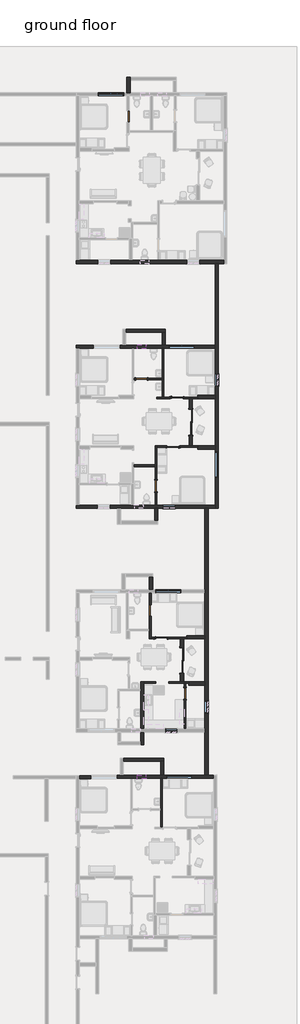
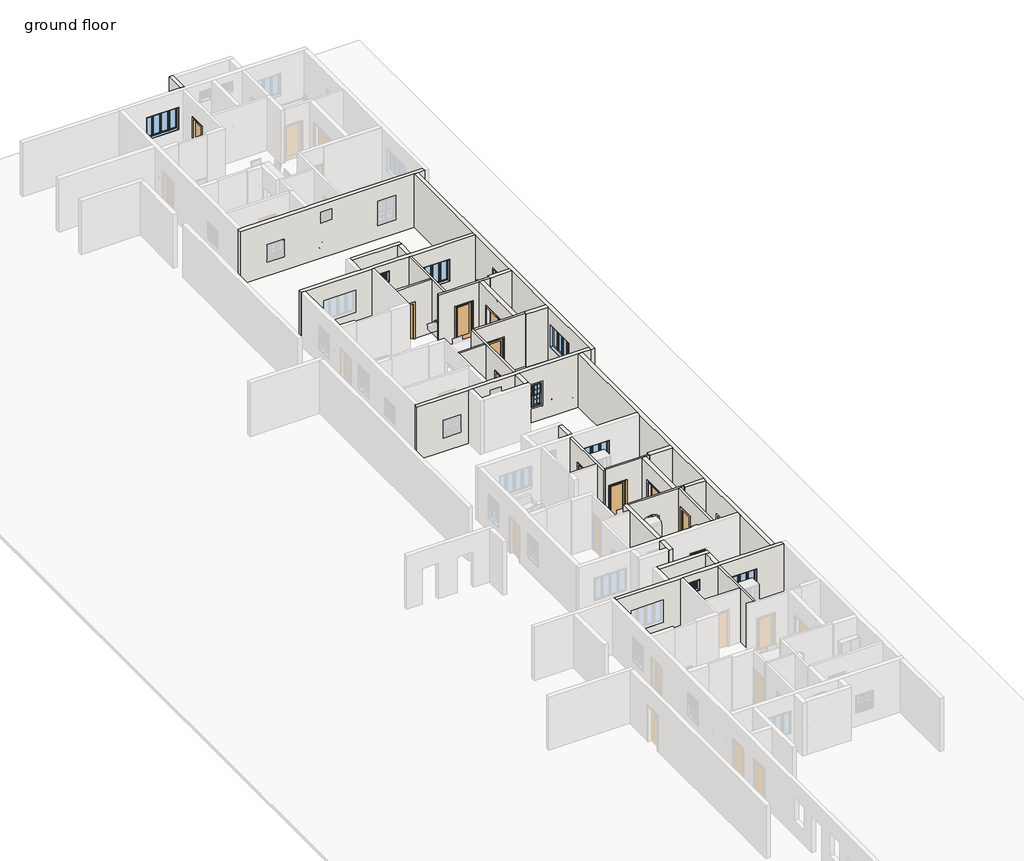
# One storey, part 9 of 16: 32 walls, 11 windows, 10 doors.
"""IFC4 building model written with IfcOpenShell, lengths in millimetres."""

from ifc_helpers import new_model, si_unit, point, frame, origin, place, context, project, spatial, polyline, ellipse_curve, trimmed, outline, extrude, faceted_brep, transform, mapped, element, save
from ifc_brep_helpers import plane_surface, extruded_surface, advanced_brep
from components import door_d4d75d1e, door_3c6ab76a, door_377e7377, door_38851409, door_d141acb4, window_ced37e8f, window_5487fb6d, window_f2d8fef0, window_45970670

model = new_model("IFC4")

# Units and contexts
model_context = context("Model", 3, world=origin())
ifc_project = project(units=[si_unit("LENGTHUNIT", "METRE", prefix="MILLI")], contexts=[model_context])

# Site, building, storey
site = spatial("IfcSite", under=ifc_project)
building = spatial("IfcBuilding", under=site)
storey = spatial("IfcBuildingStorey", under=building, Name="ground floor", Elevation=609.6)

# Doors
placement = place(None, origin())
door_shape = door_d4d75d1e(model_context)
element("IfcDoor", 1, ObjectType="Door-Double-Sliding : 72\" x 84\"", at=placement, inside=storey, context=model_context, shape_type="MappedRepresentation", body=[
    mapped(door_shape, transform((67382.9312819, 27142.5650652, 609.6), x_axis=(0.0, -1.0, 0.0), y_axis=(1.0, 0.0, 0.0), z_axis=(0.0, 0.0, 1.0))),
])
element("IfcDoor", 2, ObjectType="Door-Double-Sliding : 72\" x 84\"", at=placement, inside=storey, context=model_context, shape_type="MappedRepresentation", body=[
    mapped(door_shape, transform((66760.6312819, 10200.7650652, 609.6), x_axis=(0.0, -1.0, 0.0), y_axis=(1.0, 0.0, 0.0), z_axis=(0.0, 0.0, 1.0))),
])
door_2_shape = door_3c6ab76a(model_context)
element("IfcDoor", 3, ObjectType="Door-Interior-Single-1_Panel-Wood : 36\" x 84\"", at=placement, inside=storey, context=model_context, shape_type="MappedRepresentation", body=[
    mapped(door_2_shape, transform((66522.5062819, 28879.2900652, 609.6), x_axis=(1.0, 0.0, 0.0), y_axis=(0.0, 1.0, 0.0), z_axis=(0.0, 0.0, 1.0))),
])
element("IfcDoor", 4, ObjectType="Door-Interior-Single-1_Panel-Wood : 36\" x 84\"", at=placement, inside=storey, context=model_context, shape_type="MappedRepresentation", body=[
    mapped(door_2_shape, transform((66281.2062819, 25405.8400652, 609.6), x_axis=(-1.0, 0.0, 0.0), y_axis=(0.0, -1.0, 0.0), z_axis=(0.0, 0.0, 1.0))),
])
element("IfcDoor", 5, ObjectType="Door-Interior-Single-1_Panel-Wood : 36\" x 84\"", at=placement, inside=storey, context=model_context, shape_type="MappedRepresentation", body=[
    mapped(door_2_shape, transform((65395.3812819, 11785.0900652, 609.6), x_axis=(1.0, 0.0, 0.0), y_axis=(0.0, 1.0, 0.0), z_axis=(0.0, 0.0, 1.0))),
])
door_3_shape = door_377e7377(model_context)
element("IfcDoor", 6, ObjectType="Single-Flush : 32\" x 84\"", at=placement, inside=storey, context=model_context, shape_type="MappedRepresentation", body=[
    mapped(door_3_shape, transform((63051.0711425, 48883.2273256, 609.6), x_axis=(0.0, -1.0, 0.0), y_axis=(1.0, 0.0, 0.0), z_axis=(0.0, 0.0, 1.0))),
])
door_4_shape = door_38851409(model_context)
element("IfcDoor", 7, ObjectType="Single-Flush : 32\" x 84\"", at=placement, inside=storey, context=model_context, shape_type="MappedRepresentation", body=[
    mapped(door_4_shape, transform((67097.1812819, 7857.6150652, 609.6), x_axis=(0.0, 1.0, 0.0), y_axis=(-1.0, 0.0, 0.0), z_axis=(0.0, 0.0, 1.0))),
])
element("IfcDoor", 8, ObjectType="Single-Flush : 32\" x 84\"", at=placement, inside=storey, context=model_context, shape_type="MappedRepresentation", body=[
    mapped(door_4_shape, transform((64633.3812819, 13734.5400652, 609.6), x_axis=(0.0, -1.0, 0.0), y_axis=(1.0, 0.0, 0.0), z_axis=(0.0, 0.0, 1.0))),
])
door_5_shape = door_d141acb4(model_context)
element("IfcDoor", 9, ObjectType="Single-Flush : 32\" x 84\"", at=placement, inside=storey, context=model_context, shape_type="MappedRepresentation", body=[
    mapped(door_5_shape, transform((64023.7812819, 30209.6150652, 609.6), x_axis=(1.0, 0.0, 0.0), y_axis=(0.0, 1.0, 0.0), z_axis=(0.0, 0.0, 1.0))),
])
element("IfcDoor", 10, ObjectType="Single-Flush : 32\" x 84\"", at=placement, inside=storey, context=model_context, shape_type="MappedRepresentation", body=[
    mapped(door_5_shape, transform((65052.4812819, 22592.7900652, 609.6), x_axis=(0.0, 1.0, 0.0), y_axis=(-1.0, 0.0, 0.0), z_axis=(0.0, 0.0, 1.0))),
])

# Walls
element("IfcWall", 11, ObjectType="Generic - 4.5\"", at=placement, inside=storey, context=model_context, shape_type="SweptSolid", body=[
    extrude(outline(polyline([(64995.3312819, 23992.9650652), (63471.3312819, 23992.9650652), (63471.3312819, 24107.2650652), (64995.3312819, 24107.2650652), (64995.3312819, 23992.9650652)])), frame((0.0, 0.0, 609.6), z_axis=(0.0, 0.0, 1.0), x_axis=(1.0, 0.0, 0.0)), (0.0, 0.0, 1.0), 3200.4),
])
element("IfcWall", 12, ObjectType="Generic - 4.5\"", at=placement, inside=storey, context=model_context, shape_type="Brep", body=[
    faceted_brep([(64995.3312819, 25466.1650652, 609.6), (64995.3312819, 24107.2650652, 609.6), (64995.3312819, 23992.9650652, 609.6), (64995.3312819, 22999.1900652, 609.6), (64995.3312819, 22999.1900652, 2743.2), (64995.3312819, 22186.3900652, 2743.2), (64995.3312819, 22186.3900652, 609.6), (64995.3312819, 21249.7650652, 609.6), (64995.3312819, 21249.7650652, 3810.0), (64995.3312819, 23992.9650652, 3810.0), (64995.3312819, 24107.2650652, 3810.0), (64995.3312819, 25466.1650652, 3810.0), (65109.6312819, 22999.1900652, 2743.2), (65109.6312819, 22999.1900652, 609.6), (65109.6312819, 25351.8650652, 609.6), (65109.6312819, 25466.1650652, 609.6), (65109.6312819, 25466.1650652, 3810.0), (65109.6312819, 25351.8650652, 3810.0), (65109.6312819, 21249.7650652, 3810.0), (65109.6312819, 21249.7650652, 609.6), (65109.6312819, 22186.3900652, 609.6), (65109.6312819, 22186.3900652, 2743.2)], [[[0, 1, 2, 3, 4, 5, 6, 7, 8, 9, 10, 11]], [[12, 13, 14, 15, 16, 17, 18, 19, 20, 21]], [[20, 19, 7, 6]], [[15, 14, 13, 3, 2, 1, 0]], [[11, 10, 9, 8, 18, 17, 16]], [[8, 7, 19, 18]], [[0, 11, 16, 15]], [[4, 3, 13, 12]], [[5, 4, 12, 21]], [[6, 5, 21, 20]]]),
])
element("IfcWall", 13, ObjectType="Generic - 4.5\"", at=placement, inside=storey, context=model_context, shape_type="Brep", body=[
    faceted_brep([(68017.0909667, 25351.8650652, 609.6), (68017.0909667, 25351.8650652, 3810.0), (65109.6312819, 25351.8650652, 3810.0), (65109.6312819, 25351.8650652, 609.6), (65798.6062819, 25351.8650652, 609.6), (65798.6062819, 25351.8650652, 2768.6), (66763.8062819, 25351.8650652, 2768.6), (66763.8062819, 25351.8650652, 609.6), (68017.0909667, 25466.1650652, 3810.0), (68017.0909667, 25466.1650652, 609.6), (67624.2312819, 25466.1650652, 609.6), (67395.6312819, 25466.1650652, 609.6), (66763.8062819, 25466.1650652, 609.6), (66763.8062819, 25466.1650652, 2768.6), (65798.6062819, 25466.1650652, 2768.6), (65798.6062819, 25466.1650652, 609.6), (65109.6312819, 25466.1650652, 609.6), (65109.6312819, 25466.1650652, 3810.0), (67395.6312819, 25466.1650652, 3810.0), (67624.2312819, 25466.1650652, 3810.0)], [[[0, 1, 2, 3, 4, 5, 6, 7]], [[8, 9, 10, 11, 12, 13, 14, 15, 16, 17, 18, 19]], [[3, 16, 15, 4]], [[9, 0, 7, 12, 11, 10]], [[1, 0, 9, 8]], [[2, 1, 8, 19, 18, 17]], [[3, 2, 17, 16]], [[14, 5, 4, 15]], [[5, 14, 13, 6]], [[6, 13, 12, 7]]]),
])
element("IfcWall", 14, ObjectType="Generic - 4.5\"", at=placement, inside=storey, context=model_context, shape_type="SweptSolid", body=[
    extrude(outline(polyline([(2743.2, 64430.1812819), (609.6, 64430.1812819), (609.6, 65477.9312819), (3810.0, 65477.9312819), (3810.0, 63471.3312819), (609.6, 63471.3312819), (609.6, 63617.3812819), (2743.2, 63617.3812819), (2743.2, 64430.1812819)])), frame((0.0, 30152.4650652, 0.0), z_axis=(0.0, 1.0, 0.0), x_axis=(0.0, 0.0, 1.0)), (0.0, 0.0, 1.0), 114.3),
])
element("IfcWall", 15, ObjectType="Generic - 4.5\"", at=placement, inside=storey, context=model_context, shape_type="Brep", body=[
    faceted_brep([(65477.9312819, 32400.3650652, 609.6), (65477.9312819, 30266.7650652, 609.6), (65477.9312819, 30152.4650652, 609.6), (65477.9312819, 28933.2650652, 609.6), (65477.9312819, 28933.2650652, 3810.0), (65477.9312819, 30152.4650652, 3810.0), (65477.9312819, 30266.7650652, 3810.0), (65477.9312819, 32400.3650652, 3810.0), (65592.2312819, 32400.3650652, 609.6), (65592.2312819, 32400.3650652, 3810.0), (65592.2312819, 28933.2650652, 3810.0), (65592.2312819, 28933.2650652, 609.6)], [[[0, 1, 2, 3, 4, 5, 6, 7]], [[8, 9, 10, 11]], [[3, 2, 1, 0, 8, 11]], [[7, 6, 5, 4, 10, 9]], [[0, 7, 9, 8]], [[4, 3, 11, 10]]]),
])
element("IfcWall", 16, ObjectType="Generic - 4.5\"", at=placement, inside=storey, context=model_context, shape_type="Brep", body=[
    faceted_brep([(68017.0909667, 28818.9650652, 609.6), (68017.0909667, 28818.9650652, 3810.0), (67624.2312819, 28818.9650652, 3810.0), (67395.6312819, 28818.9650652, 3810.0), (65109.6312819, 28818.9650652, 3810.0), (65109.6312819, 28818.9650652, 609.6), (66039.9062819, 28818.9650652, 609.6), (66039.9062819, 28818.9650652, 2768.6), (67005.1062819, 28818.9650652, 2768.6), (67005.1062819, 28818.9650652, 609.6), (67395.6312819, 28818.9650652, 609.6), (67624.2312819, 28818.9650652, 609.6), (68017.0909667, 28933.2650652, 3810.0), (68017.0909667, 28933.2650652, 609.6), (67005.1062819, 28933.2650652, 609.6), (67005.1062819, 28933.2650652, 2768.6), (66039.9062819, 28933.2650652, 2768.6), (66039.9062819, 28933.2650652, 609.6), (65592.2312819, 28933.2650652, 609.6), (65477.9312819, 28933.2650652, 609.6), (65109.6312819, 28933.2650652, 609.6), (65109.6312819, 28933.2650652, 3810.0), (65477.9312819, 28933.2650652, 3810.0), (65592.2312819, 28933.2650652, 3810.0)], [[[0, 1, 2, 3, 4, 5, 6, 7, 8, 9, 10, 11]], [[12, 13, 14, 15, 16, 17, 18, 19, 20, 21, 22, 23]], [[5, 20, 19, 18, 17, 6]], [[13, 0, 11, 10, 9, 14]], [[1, 0, 13, 12]], [[4, 3, 2, 1, 12, 23, 22, 21]], [[5, 4, 21, 20]], [[8, 15, 14, 9]], [[15, 8, 7, 16]], [[16, 7, 6, 17]]]),
])
element("IfcWall", 17, ObjectType="Generic - 4.5\"", at=placement, inside=storey, context=model_context, shape_type="Brep", body=[
    faceted_brep([(64576.2312819, 13328.1400652, 2743.2), (64576.2312819, 13328.1400652, 609.6), (64576.2312819, 12410.5650652, 609.6), (64576.2312819, 12296.2650652, 609.6), (64576.2312819, 11724.7650652, 609.6), (64576.2312819, 11724.7650652, 3810.0), (64576.2312819, 12296.2650652, 3810.0), (64576.2312819, 12410.5650652, 3810.0), (64576.2312819, 15001.3650652, 3810.0), (64576.2312819, 15001.3650652, 609.6), (64576.2312819, 14140.9400652, 609.6), (64576.2312819, 14140.9400652, 2743.2), (64690.5312819, 11724.7650652, 609.6), (64690.5312819, 11839.0650652, 609.6), (64690.5312819, 13328.1400652, 609.6), (64690.5312819, 13328.1400652, 2743.2), (64690.5312819, 14140.9400652, 2743.2), (64690.5312819, 14140.9400652, 609.6), (64690.5312819, 15001.3650652, 609.6), (64690.5312819, 15001.3650652, 3810.0), (64690.5312819, 11839.0650652, 3810.0), (64690.5312819, 11724.7650652, 3810.0)], [[[0, 1, 2, 3, 4, 5, 6, 7, 8, 9, 10, 11]], [[12, 13, 14, 15, 16, 17, 18, 19, 20, 21]], [[10, 9, 18, 17]], [[4, 3, 2, 1, 14, 13, 12]], [[8, 7, 6, 5, 21, 20, 19]], [[9, 8, 19, 18]], [[5, 4, 12, 21]], [[15, 14, 1, 0]], [[16, 15, 0, 11]], [[17, 16, 11, 10]]]),
])
element("IfcWall", 18, ObjectType="Generic - 4.5\"", at=placement, inside=storey, context=model_context, shape_type="Brep", body=[
    faceted_brep([(67216.0628293, 11724.7650652, 609.6), (67216.0628293, 11724.7650652, 3810.0), (67001.9312819, 11724.7650652, 3810.0), (66773.3312819, 11724.7650652, 3810.0), (64690.5312819, 11724.7650652, 3810.0), (64690.5312819, 11724.7650652, 609.6), (64912.7812819, 11724.7650652, 609.6), (64912.7812819, 11724.7650652, 2768.6), (65877.9812819, 11724.7650652, 2768.6), (65877.9812819, 11724.7650652, 609.6), (66773.3312819, 11724.7650652, 609.6), (67001.9312819, 11724.7650652, 609.6), (67216.0628293, 11839.0650652, 3810.0), (67216.0628293, 11839.0650652, 609.6), (65877.9812819, 11839.0650652, 609.6), (65877.9812819, 11839.0650652, 2768.6), (64912.7812819, 11839.0650652, 2768.6), (64912.7812819, 11839.0650652, 609.6), (64690.5312819, 11839.0650652, 609.6), (64690.5312819, 11839.0650652, 3810.0)], [[[0, 1, 2, 3, 4, 5, 6, 7, 8, 9, 10, 11]], [[12, 13, 14, 15, 16, 17, 18, 19]], [[5, 18, 17, 6]], [[13, 0, 11, 10, 9, 14]], [[1, 0, 13, 12]], [[4, 3, 2, 1, 12, 19]], [[5, 4, 19, 18]], [[8, 15, 14, 9]], [[15, 8, 7, 16]], [[16, 7, 6, 17]]]),
])
element("IfcWall", 19, ObjectType="Generic - 4.5\"", at=placement, inside=storey, context=model_context, shape_type="AdvancedBrep", body=[
    advanced_brep(
    [(65020.7312819, 8676.7650652, 2540.0), (65020.7312819, 8676.7650652, 609.6), (64182.5312819, 8676.7650652, 609.6), (64182.5312819, 8676.7650652, 3810.0), (66773.3312819, 8676.7650652, 3810.0), (67001.9312819, 8676.7650652, 3810.0), (67357.5312819, 8676.7650652, 3810.0), (67357.5312819, 8676.7650652, 609.6), (67001.9312819, 8676.7650652, 609.6), (66773.3312819, 8676.7650652, 609.6), (65935.1312819, 8676.7650652, 609.6), (65935.1312819, 8676.7650652, 2540.0), (64182.5312819, 8562.4650652, 609.6), (65020.7312819, 8562.4650652, 609.6), (65020.7312819, 8562.4650652, 2540.0), (65935.1312819, 8562.4650652, 2540.0), (65935.1312819, 8562.4650652, 609.6), (67040.0312819, 8562.4650652, 609.6), (67154.3312819, 8562.4650652, 609.6), (67357.5312819, 8562.4650652, 609.6), (67357.5312819, 8562.4650652, 3810.0), (67154.3312819, 8562.4650652, 3810.0), (67040.0312819, 8562.4650652, 3810.0), (64182.5312819, 8562.4650652, 3810.0)],
    [
        (0, 1),
        (1, 2),
        (2, 3),
        (3, 4),
        (4, 5),
        (5, 6),
        (6, 7),
        (7, 8),
        (8, 9),
        (9, 10),
        (10, 11),
        (11, 0, ellipse_curve(frame((65477.9312819, 8676.7650652, 2540.0), z_axis=(0.0, -1.0, 0.0), x_axis=(-1.0, 0.0, 0.0)), 457.2, 203.2)),
        (12, 13),
        (13, 14),
        (14, 15, ellipse_curve(frame((65477.9312819, 8562.4650652, 2540.0), z_axis=(0.0, 1.0, 0.0), x_axis=(-1.0, 0.0, 0.0)), 457.2, 203.2)),
        (15, 16),
        (16, 17),
        (17, 18),
        (18, 19),
        (19, 20),
        (20, 21),
        (21, 22),
        (22, 23),
        (23, 12),
        (1, 13),
        (12, 2),
        (7, 19),
        (16, 10),
        (3, 23),
        (20, 6),
        (14, 0),
        (11, 15),
    ],
    [
        plane_surface(frame((67354.7375714, 8676.7650652, 609.6), z_axis=(0.0, 1.0, 0.0), x_axis=(-1.0, 0.0, 0.0))),
        plane_surface(frame((67354.7375714, 8562.4650652, 609.6), z_axis=(0.0, -1.0, 0.0), x_axis=(1.0, 0.0, 0.0))),
        plane_surface(frame((67357.5312819, 8676.7650652, 609.6), z_axis=(0.0, 0.0, -1.0), x_axis=(0.0, -1.0, 0.0))),
        plane_surface(frame((64068.2312819, 8676.7650652, 3810.0), z_axis=(0.0, 0.0, 1.0), x_axis=(0.0, -1.0, 0.0))),
        plane_surface(frame((67357.5312819, 8676.7650652, 3810.0), z_axis=(1.0, 0.0, 0.0), x_axis=(0.0, -1.0, 0.0))),
        plane_surface(frame((64182.5312819, 8663.9647578, 609.6), z_axis=(-1.0, 0.0, 0.0), x_axis=(0.0, 1.0, 0.0))),
        extruded_surface(trimmed(ellipse_curve(frame((65477.9312819, 8791.0650652, 2540.0), z_axis=(0.0, 1.0, 0.0), x_axis=(-1.0, 0.0, 0.0)), 457.2, 203.2), [point((65020.7312819, 8791.0650652, 2540.0))], [point((65935.1312819, 8791.0650652, 2540.0))], True, "CARTESIAN"), (0.0, -114.30000000000109, 0.0), 114.30000000000109),
        plane_surface(frame((65935.1312819, 8562.4650652, 2540.0), z_axis=(-1.0, 0.0, 0.0), x_axis=(0.0, 1.0, 0.0))),
        plane_surface(frame((65020.7312819, 8562.4650652, 609.6), z_axis=(1.0, 0.0, 0.0), x_axis=(0.0, 1.0, 0.0))),
    ],
    [
        (0, [[1, 2, 3, 4, 5, 6, 7, 8, 9, 10, 11, 12]]),
        (1, [[13, 14, 15, 16, 17, 18, 19, 20, 21, 22, 23, 24]]),
        (2, [[-2, 25, -13, 26]]),
        (2, [[-10, -9, -8, 27, -19, -18, -17, 28]]),
        (3, [[-6, -5, -4, 29, -23, -22, -21, 30]]),
        (4, [[-7, -30, -20, -27]]),
        (5, [[-3, -26, -24, -29]]),
        (6, [[-15, 31, -12, 32]]),
        (7, [[-16, -32, -11, -28]]),
        (8, [[-14, -25, -1, -31]]),
    ],
),
])
element("IfcWall", 20, ObjectType="Generic - 4.5\"", at=placement, inside=storey, context=model_context, shape_type="SweptSolid", body=[
    extrude(outline(polyline([(8562.4650652, 609.6), (8264.0150652, 609.6), (8264.0150652, 2743.2), (7451.2150652, 2743.2), (7451.2150652, 609.6), (5323.9650652, 609.6), (5323.9650652, 3810.0), (8562.4650652, 3810.0), (8562.4650652, 609.6)])), frame((67040.0312819, 0.0, 0.0), z_axis=(1.0, 0.0, 0.0), x_axis=(0.0, 1.0, 0.0)), (0.0, 0.0, 1.0), 114.3),
])
element("IfcWall", 21, ObjectType="Generic - 4.5\"", at=placement, inside=storey, context=model_context, shape_type="Brep", body=[
    faceted_brep([(65363.6312819, 1802.356101, 609.6), (65363.6312819, -346.8113664, 609.6), (65363.6312819, -461.1113664, 609.6), (65363.6312819, -1680.3113664, 609.6), (65363.6312819, -1680.3113664, 3810.0), (65363.6312819, -461.1113664, 3810.0), (65363.6312819, -346.8113664, 3810.0), (65363.6312819, 1802.356101, 3810.0), (65477.9312819, 1802.8108651, 609.6), (65477.9312819, 1802.8108651, 3810.0), (65477.9312819, -1680.3113664, 3810.0), (65477.9312819, -1680.3113664, 609.6)], [[[0, 1, 2, 3, 4, 5, 6, 7]], [[8, 9, 10, 11]], [[3, 2, 1, 0, 8, 11]], [[7, 6, 5, 4, 10, 9]], [[0, 7, 9, 8]], [[4, 3, 11, 10]]]),
])
element("IfcWall", 22, ObjectType="Generic - 9\"", at=placement, inside=storey, context=model_context, shape_type="Brep", body=[
    faceted_brep([(69856.4363207, 38662.1809867, 609.6), (65285.5257323, 38662.1809867, 609.6), (65171.2257323, 38662.1809867, 609.6), (63351.5731635, 38662.1809867, 609.6), (63148.3731635, 38662.1809867, 609.6), (59585.1312819, 38662.1809867, 609.6), (59356.5312819, 38662.1809867, 609.6), (59356.5312819, 38662.1809867, 3810.0), (59585.1312819, 38662.1809867, 3810.0), (63148.3731635, 38662.1809867, 3810.0), (63351.5731635, 38662.1809867, 3810.0), (65171.2257323, 38662.1809867, 3810.0), (65285.5257323, 38662.1809867, 3810.0), (69856.4363207, 38662.1809867, 3810.0), (68144.9312819, 38662.1809867, 2844.8), (67230.5312819, 38662.1809867, 2844.8), (67230.5312819, 38662.1809867, 1524.0), (68144.9312819, 38662.1809867, 1524.0), (60928.6022227, 38662.1809867, 2438.4), (60928.6022227, 38662.1809867, 1524.0), (61792.2022227, 38662.1809867, 1524.0), (61792.2022227, 38662.1809867, 2438.4), (64543.9744479, 38662.1809867, 3352.8), (63934.3744479, 38662.1809867, 3352.8), (63934.3744479, 38662.1809867, 2743.2), (64543.9744479, 38662.1809867, 2743.2), (69856.4363207, 38433.5809867, 609.6), (69856.4363207, 38433.5809867, 3810.0), (69478.4312819, 38433.5809867, 3810.0), (69249.8312819, 38433.5809867, 3810.0), (59356.5312819, 38433.5809867, 3810.0), (59356.5312819, 38433.5809867, 609.6), (69249.8312819, 38433.5809867, 609.6), (69478.4312819, 38433.5809867, 609.6), (68144.9312819, 38433.5809867, 2844.8), (68144.9312819, 38433.5809867, 1524.0), (67230.5312819, 38433.5809867, 1524.0), (67230.5312819, 38433.5809867, 2844.8), (60928.6022227, 38433.5809867, 2438.4), (61792.2022227, 38433.5809867, 2438.4), (61792.2022227, 38433.5809867, 1524.0), (60928.6022227, 38433.5809867, 1524.0), (64543.9744479, 38433.5809867, 3352.8), (64543.9744479, 38433.5809867, 2743.2), (63934.3744479, 38433.5809867, 2743.2), (63934.3744479, 38433.5809867, 3352.8)], [[[0, 1, 2, 3, 4, 5, 6, 7, 8, 9, 10, 11, 12, 13], [14, 15, 16, 17], [18, 19, 20, 21], [22, 23, 24, 25]], [[26, 27, 28, 29, 30, 31, 32, 33], [34, 35, 36, 37], [38, 39, 40, 41], [42, 43, 44, 45]], [[6, 5, 4, 3, 2, 1, 0, 26, 33, 32, 31]], [[13, 12, 11, 10, 9, 8, 7, 30, 29, 28, 27]], [[0, 13, 27, 26]], [[7, 6, 31, 30]], [[35, 34, 14, 17]], [[36, 35, 17, 16]], [[37, 36, 16, 15]], [[34, 37, 15, 14]], [[19, 18, 38, 41]], [[20, 19, 41, 40]], [[21, 20, 40, 39]], [[18, 21, 39, 38]], [[43, 42, 22, 25]], [[44, 43, 25, 24]], [[45, 44, 24, 23]], [[42, 45, 23, 22]]]),
])
element("IfcWall", 23, ObjectType="Generic - 9\"", at=placement, inside=storey, context=model_context, shape_type="Brep", body=[
    faceted_brep([(63196.436417, 50583.0390836, 609.6), (63196.436417, 51470.3211687, 609.6), (63196.436417, 51698.9211687, 609.6), (63196.436417, 51698.9211687, 3810.0), (63196.436417, 51470.3211687, 3810.0), (63196.436417, 50583.0390836, 3810.0), (62967.836417, 50583.0390836, 609.6), (62967.836417, 50583.0390836, 3810.0), (62967.836417, 51698.9211687, 3810.0), (62967.836417, 51698.9211687, 609.6)], [[[0, 1, 2, 3, 4, 5]], [[6, 7, 8, 9]], [[2, 1, 0, 6, 9]], [[5, 4, 3, 8, 7]], [[0, 5, 7, 6]], [[3, 2, 9, 8]]]),
])
element("IfcWall", 24, ObjectType="Generic - 9\"", at=placement, inside=storey, context=model_context, shape_type="Brep", body=[
    faceted_brep([(59356.5312819, 32400.3650652, 609.6), (59585.1312819, 32400.3650652, 609.6), (63357.0312819, 32400.3650652, 609.6), (63471.3312819, 32400.3650652, 609.6), (65477.9312819, 32400.3650652, 609.6), (65592.2312819, 32400.3650652, 609.6), (69249.8312819, 32400.3650652, 609.6), (69249.8312819, 32400.3650652, 3810.0), (65592.2312819, 32400.3650652, 3810.0), (65477.9312819, 32400.3650652, 3810.0), (63471.3312819, 32400.3650652, 3810.0), (63357.0312819, 32400.3650652, 3810.0), (59585.1312819, 32400.3650652, 3810.0), (59356.5312819, 32400.3650652, 3810.0), (62447.8192161, 32400.3650652, 2870.2), (62447.8192161, 32400.3650652, 1524.0), (60619.0192161, 32400.3650652, 1524.0), (60619.0192161, 32400.3650652, 2870.2), (67776.6312819, 32400.3650652, 2870.2), (67776.6312819, 32400.3650652, 1524.0), (65947.8312819, 32400.3650652, 1524.0), (65947.8312819, 32400.3650652, 2870.2), (63718.9812819, 32400.3650652, 3352.8), (64328.5812819, 32400.3650652, 3352.8), (64328.5812819, 32400.3650652, 2743.2), (63718.9812819, 32400.3650652, 2743.2), (59356.5312819, 32628.9650652, 609.6), (59356.5312819, 32628.9650652, 3810.0), (62663.7192161, 32628.9650652, 3810.0), (62892.3192161, 32628.9650652, 3810.0), (65477.9312819, 32628.9650652, 3810.0), (65706.5312819, 32628.9650652, 3810.0), (69249.8312819, 32628.9650652, 3810.0), (69249.8312819, 32628.9650652, 609.6), (65706.5312819, 32628.9650652, 609.6), (65477.9312819, 32628.9650652, 609.6), (62892.3192161, 32628.9650652, 609.6), (62663.7192161, 32628.9650652, 609.6), (62447.8192161, 32628.9650652, 2870.2), (60619.0192161, 32628.9650652, 2870.2), (60619.0192161, 32628.9650652, 1524.0), (62447.8192161, 32628.9650652, 1524.0), (67776.6312819, 32628.9650652, 2870.2), (65947.8312819, 32628.9650652, 2870.2), (65947.8312819, 32628.9650652, 1524.0), (67776.6312819, 32628.9650652, 1524.0), (63718.9812819, 32628.9650652, 3352.8), (63718.9812819, 32628.9650652, 2743.2), (64328.5812819, 32628.9650652, 2743.2), (64328.5812819, 32628.9650652, 3352.8)], [[[0, 1, 2, 3, 4, 5, 6, 7, 8, 9, 10, 11, 12, 13], [14, 15, 16, 17], [18, 19, 20, 21], [22, 23, 24, 25]], [[26, 27, 28, 29, 30, 31, 32, 33, 34, 35, 36, 37], [38, 39, 40, 41], [42, 43, 44, 45], [46, 47, 48, 49]], [[6, 5, 4, 3, 2, 1, 0, 26, 37, 36, 35, 34, 33]], [[13, 12, 11, 10, 9, 8, 7, 32, 31, 30, 29, 28, 27]], [[7, 6, 33, 32]], [[0, 13, 27, 26]], [[15, 14, 38, 41]], [[16, 15, 41, 40]], [[17, 16, 40, 39]], [[14, 17, 39, 38]], [[19, 18, 42, 45]], [[20, 19, 45, 44]], [[21, 20, 44, 43]], [[18, 21, 43, 42]], [[47, 46, 22, 25]], [[48, 47, 25, 24]], [[49, 48, 24, 23]], [[46, 49, 23, 22]]]),
])
element("IfcWall", 25, ObjectType="Generic - 9\"", at=placement, inside=storey, context=model_context, shape_type="Brep", body=[
    faceted_brep([(69249.8312819, 38433.5809867, 609.6), (69249.8312819, 32628.9650652, 609.6), (69249.8312819, 32400.3650652, 609.6), (69249.8312819, 29047.5650652, 609.6), (69249.8312819, 28818.9650652, 609.6), (69249.8312819, 25466.1650652, 609.6), (69249.8312819, 25237.5650652, 609.6), (69249.8312819, 21249.7650652, 609.6), (69249.8312819, 21021.1650652, 609.6), (69249.8312819, 21021.1650652, 3810.0), (69249.8312819, 21249.7650652, 3810.0), (69249.8312819, 25237.5650652, 3810.0), (69249.8312819, 25466.1650652, 3810.0), (69249.8312819, 28818.9650652, 3810.0), (69249.8312819, 29047.5650652, 3810.0), (69249.8312819, 32400.3650652, 3810.0), (69249.8312819, 32628.9650652, 3810.0), (69249.8312819, 38433.5809867, 3810.0), (69249.8312819, 23218.2650652, 2870.2), (69249.8312819, 23218.2650652, 1524.0), (69249.8312819, 25047.0650652, 1524.0), (69249.8312819, 25047.0650652, 2870.2), (69249.8312819, 30609.6650652, 2844.8), (69249.8312819, 29695.2650652, 2844.8), (69249.8312819, 29695.2650652, 1524.0), (69249.8312819, 30609.6650652, 1524.0), (69478.4312819, 38433.5809867, 609.6), (69478.4312819, 38433.5809867, 3810.0), (69478.4312819, 21021.1650652, 3810.0), (69478.4312819, 21021.1650652, 609.6), (69478.4312819, 23218.2650652, 2870.2), (69478.4312819, 25047.0650652, 2870.2), (69478.4312819, 25047.0650652, 1524.0), (69478.4312819, 23218.2650652, 1524.0), (69478.4312819, 30609.6650652, 2844.8), (69478.4312819, 30609.6650652, 1524.0), (69478.4312819, 29695.2650652, 1524.0), (69478.4312819, 29695.2650652, 2844.8)], [[[0, 1, 2, 3, 4, 5, 6, 7, 8, 9, 10, 11, 12, 13, 14, 15, 16, 17], [18, 19, 20, 21], [22, 23, 24, 25]], [[26, 27, 28, 29], [30, 31, 32, 33], [34, 35, 36, 37]], [[8, 7, 6, 5, 4, 3, 2, 1, 0, 26, 29]], [[17, 16, 15, 14, 13, 12, 11, 10, 9, 28, 27]], [[9, 8, 29, 28]], [[0, 17, 27, 26]], [[19, 18, 30, 33]], [[20, 19, 33, 32]], [[21, 20, 32, 31]], [[18, 21, 31, 30]], [[35, 34, 22, 25]], [[36, 35, 25, 24]], [[37, 36, 24, 23]], [[34, 37, 23, 22]]]),
])
element("IfcWall", 26, ObjectType="Generic - 9\"", at=placement, inside=storey, context=model_context, shape_type="Brep", body=[
    faceted_brep([(69249.8312819, 21249.7650652, 609.6), (65109.6312819, 21249.7650652, 609.6), (64995.3312819, 21249.7650652, 609.6), (63471.3312819, 21249.7650652, 609.6), (63268.1312819, 21249.7650652, 609.6), (59585.1312819, 21249.7650652, 609.6), (59356.5312819, 21249.7650652, 609.6), (59356.5312819, 21249.7650652, 3810.0), (59585.1312819, 21249.7650652, 3810.0), (63268.1312819, 21249.7650652, 3810.0), (63471.3312819, 21249.7650652, 3810.0), (64995.3312819, 21249.7650652, 3810.0), (65109.6312819, 21249.7650652, 3810.0), (69249.8312819, 21249.7650652, 3810.0), (66429.5983059, 21249.7650652, 2844.8), (65515.1983059, 21249.7650652, 2844.8), (65515.1983059, 21249.7650652, 1524.0), (66429.5983059, 21249.7650652, 1524.0), (60905.9312819, 21249.7650652, 2438.4), (60905.9312819, 21249.7650652, 1524.0), (61769.5312819, 21249.7650652, 1524.0), (61769.5312819, 21249.7650652, 2438.4), (64131.7312819, 21249.7650652, 3352.8), (63522.1312819, 21249.7650652, 3352.8), (63522.1312819, 21249.7650652, 2743.2), (64131.7312819, 21249.7650652, 2743.2), (69249.8312819, 21021.1650652, 609.6), (69249.8312819, 21021.1650652, 3810.0), (68754.5312819, 21021.1650652, 3810.0), (68525.9312819, 21021.1650652, 3810.0), (65172.2983059, 21021.1650652, 3810.0), (64943.6983059, 21021.1650652, 3810.0), (62518.8312819, 21021.1650652, 3810.0), (62290.2312819, 21021.1650652, 3810.0), (59356.5312819, 21021.1650652, 3810.0), (59356.5312819, 21021.1650652, 609.6), (62290.2312819, 21021.1650652, 609.6), (62518.8312819, 21021.1650652, 609.6), (64943.6983059, 21021.1650652, 609.6), (65172.2983059, 21021.1650652, 609.6), (68525.9312819, 21021.1650652, 609.6), (68754.5312819, 21021.1650652, 609.6), (66429.5983059, 21021.1650652, 2844.8), (66429.5983059, 21021.1650652, 1524.0), (65515.1983059, 21021.1650652, 1524.0), (65515.1983059, 21021.1650652, 2844.8), (60905.9312819, 21021.1650652, 2438.4), (61769.5312819, 21021.1650652, 2438.4), (61769.5312819, 21021.1650652, 1524.0), (60905.9312819, 21021.1650652, 1524.0), (64131.7312819, 21021.1650652, 3352.8), (64131.7312819, 21021.1650652, 2743.2), (63522.1312819, 21021.1650652, 2743.2), (63522.1312819, 21021.1650652, 3352.8)], [[[0, 1, 2, 3, 4, 5, 6, 7, 8, 9, 10, 11, 12, 13], [14, 15, 16, 17], [18, 19, 20, 21], [22, 23, 24, 25]], [[26, 27, 28, 29, 30, 31, 32, 33, 34, 35, 36, 37, 38, 39, 40, 41], [42, 43, 44, 45], [46, 47, 48, 49], [50, 51, 52, 53]], [[6, 5, 4, 3, 2, 1, 0, 26, 41, 40, 39, 38, 37, 36, 35]], [[13, 12, 11, 10, 9, 8, 7, 34, 33, 32, 31, 30, 29, 28, 27]], [[0, 13, 27, 26]], [[7, 6, 35, 34]], [[43, 42, 14, 17]], [[44, 43, 17, 16]], [[45, 44, 16, 15]], [[42, 45, 15, 14]], [[19, 18, 46, 49]], [[20, 19, 49, 48]], [[21, 20, 48, 47]], [[18, 21, 47, 46]], [[51, 50, 22, 25]], [[52, 51, 25, 24]], [[53, 52, 24, 23]], [[50, 53, 23, 22]]]),
])
element("IfcWall", 27, ObjectType="Generic - 9\"", at=placement, inside=storey, context=model_context, shape_type="Brep", body=[
    faceted_brep([(68017.0909667, 28818.9650652, 609.6), (69249.8312819, 28818.9650652, 609.6), (69249.8312819, 28818.9650652, 3810.0), (68017.0909667, 28818.9650652, 3810.0), (68017.0909667, 29047.5650652, 609.6), (68017.0909667, 29047.5650652, 3810.0), (69249.8312819, 29047.5650652, 3810.0), (69249.8312819, 29047.5650652, 609.6), (68017.0909667, 28933.2650652, 609.6), (68017.0909667, 28933.2650652, 3810.0)], [[[0, 1, 2, 3]], [[4, 5, 6, 7]], [[1, 0, 8, 4, 7]], [[3, 2, 6, 5, 9]], [[0, 3, 9, 5, 4, 8]], [[2, 1, 7, 6]]]),
])
element("IfcWall", 28, ObjectType="Generic - 9\"", at=placement, inside=storey, context=model_context, shape_type="SweptSolid", body=[
    extrude(outline(polyline([(26228.1650652, 2743.2), (26228.1650652, 609.6), (25466.1650652, 609.6), (25466.1650652, 3810.0), (28818.9650652, 3810.0), (28818.9650652, 609.6), (28056.9650652, 609.6), (28056.9650652, 2743.2), (26228.1650652, 2743.2)])), frame((67395.6312819, 0.0, 0.0), z_axis=(1.0, 0.0, 0.0), x_axis=(0.0, 1.0, 0.0)), (0.0, 0.0, 1.0), 228.6),
])
element("IfcWall", 29, ObjectType="Generic - 9\"", at=placement, inside=storey, context=model_context, shape_type="Brep", body=[
    faceted_brep([(69249.8312819, 25466.1650652, 609.6), (68017.0909667, 25466.1650652, 609.6), (68017.0909667, 25466.1650652, 3810.0), (69249.8312819, 25466.1650652, 3810.0), (69249.8312819, 25237.5650652, 609.6), (69249.8312819, 25237.5650652, 3810.0), (68017.0909667, 25237.5650652, 3810.0), (68017.0909667, 25237.5650652, 609.6), (68017.0909667, 25351.8650652, 609.6), (68017.0909667, 25351.8650652, 3810.0)], [[[0, 1, 2, 3]], [[4, 5, 6, 7]], [[1, 0, 4, 7, 8]], [[2, 1, 8, 7, 6, 9]], [[3, 2, 9, 6, 5]], [[0, 3, 5, 4]]]),
])
element("IfcWall", 30, ObjectType="Generic - 9\"", at=placement, inside=storey, context=model_context, shape_type="Brep", body=[
    faceted_brep([(62892.3192161, 33536.3470746, 609.6), (65477.9312819, 33536.3470746, 609.6), (65706.5312819, 33536.3470746, 609.6), (65706.5312819, 33536.3470746, 3810.0), (65477.9312819, 33536.3470746, 3810.0), (62892.3192161, 33536.3470746, 3810.0), (62892.3192161, 33764.9470746, 609.6), (62892.3192161, 33764.9470746, 3810.0), (65706.5312819, 33764.9470746, 3810.0), (65706.5312819, 33764.9470746, 609.6)], [[[0, 1, 2, 3, 4, 5]], [[6, 7, 8, 9]], [[2, 1, 0, 6, 9]], [[5, 4, 3, 8, 7]], [[0, 5, 7, 6]], [[3, 2, 9, 8]]]),
])
element("IfcWall", 31, ObjectType="Generic - 9\"", at=placement, inside=storey, context=model_context, shape_type="SweptSolid", body=[
    extrude(outline(polyline([(65477.9312819, 32628.9650652), (65477.9312819, 33536.3470746), (65706.5312819, 33536.3470746), (65706.5312819, 32628.9650652), (65477.9312819, 32628.9650652)])), frame((0.0, 0.0, 609.6), z_axis=(0.0, 0.0, 1.0), x_axis=(1.0, 0.0, 0.0)), (0.0, 0.0, 1.0), 3200.4),
])
element("IfcWall", 32, ObjectType="Generic - 9\"", at=placement, inside=storey, context=model_context, shape_type="SweptSolid", body=[
    extrude(outline(polyline([(65172.2983059, 21021.1650652), (65172.2983059, 20123.9539393), (64943.6983059, 20123.9539393), (64943.6983059, 21021.1650652), (65172.2983059, 21021.1650652)])), frame((0.0, 0.0, 609.6), z_axis=(0.0, 0.0, 1.0), x_axis=(1.0, 0.0, 0.0)), (0.0, 0.0, 1.0), 3200.4),
])
element("IfcWall", 33, ObjectType="Generic - 9\"", at=placement, inside=storey, context=model_context, shape_type="Brep", body=[
    faceted_brep([(68525.9312819, 21021.1650652, 609.6), (68525.9312819, 15229.9650652, 609.6), (68525.9312819, 15001.3650652, 609.6), (68525.9312819, 11953.3650652, 609.6), (68525.9312819, 11724.7650652, 609.6), (68525.9312819, 8676.7650652, 609.6), (68525.9312819, 8448.1650652, 609.6), (68525.9312819, 5323.9650652, 609.6), (68525.9312819, 5095.3650652, 609.6), (68525.9312819, 2043.5397185, 609.6), (68525.9312819, 2043.5397185, 3810.0), (68525.9312819, 5095.3650652, 3810.0), (68525.9312819, 5323.9650652, 3810.0), (68525.9312819, 8448.1650652, 3810.0), (68525.9312819, 8676.7650652, 3810.0), (68525.9312819, 11724.7650652, 3810.0), (68525.9312819, 11953.3650652, 3810.0), (68525.9312819, 15001.3650652, 3810.0), (68525.9312819, 15229.9650652, 3810.0), (68525.9312819, 21021.1650652, 3810.0), (68525.9312819, 6454.2650652, 2438.4), (68525.9312819, 6454.2650652, 1524.0), (68525.9312819, 7317.8650652, 1524.0), (68525.9312819, 7317.8650652, 2438.4), (68754.5312819, 21021.1650652, 609.6), (68754.5312819, 21021.1650652, 3810.0), (68754.5312819, 2044.4492469, 3810.0), (68754.5312819, 2044.4492469, 609.6), (68754.5312819, 6454.2650652, 2438.4), (68754.5312819, 7317.8650652, 2438.4), (68754.5312819, 7317.8650652, 1524.0), (68754.5312819, 6454.2650652, 1524.0)], [[[0, 1, 2, 3, 4, 5, 6, 7, 8, 9, 10, 11, 12, 13, 14, 15, 16, 17, 18, 19], [20, 21, 22, 23]], [[24, 25, 26, 27], [28, 29, 30, 31]], [[9, 8, 7, 6, 5, 4, 3, 2, 1, 0, 24, 27]], [[19, 18, 17, 16, 15, 14, 13, 12, 11, 10, 26, 25]], [[0, 19, 25, 24]], [[10, 9, 27, 26]], [[21, 20, 28, 31]], [[22, 21, 31, 30]], [[23, 22, 30, 29]], [[20, 23, 29, 28]]]),
])
element("IfcWall", 34, ObjectType="Generic - 9\"", at=placement, inside=storey, context=model_context, shape_type="SweptSolid", body=[
    extrude(outline(polyline([(9286.3650652, 2743.2), (9286.3650652, 609.6), (8676.7650652, 609.6), (8676.7650652, 3810.0), (11724.7650652, 3810.0), (11724.7650652, 609.6), (11115.1650652, 609.6), (11115.1650652, 2743.2), (9286.3650652, 2743.2)])), frame((66773.3312819, 0.0, 0.0), z_axis=(1.0, 0.0, 0.0), x_axis=(0.0, 1.0, 0.0)), (0.0, 0.0, 1.0), 228.6),
])
element("IfcWall", 35, ObjectType="Generic - 9\"", at=placement, inside=storey, context=model_context, shape_type="Brep", body=[
    faceted_brep([(67216.0628293, 11724.7650652, 609.6), (68525.9312819, 11724.7650652, 609.6), (68525.9312819, 11724.7650652, 3810.0), (67216.0628293, 11724.7650652, 3810.0), (67216.0628293, 11953.3650652, 609.6), (67216.0628293, 11953.3650652, 3810.0), (68525.9312819, 11953.3650652, 3810.0), (68525.9312819, 11953.3650652, 609.6), (67216.0628293, 11839.0650652, 609.6), (67216.0628293, 11839.0650652, 3810.0)], [[[0, 1, 2, 3]], [[4, 5, 6, 7]], [[1, 0, 8, 4, 7]], [[3, 2, 6, 5, 9]], [[0, 3, 9, 5, 4, 8]], [[2, 1, 7, 6]]]),
])
element("IfcWall", 36, ObjectType="Generic - 9\"", at=placement, inside=storey, context=model_context, shape_type="Brep", body=[
    faceted_brep([(68525.9312819, 8676.7650652, 609.6), (67357.5312819, 8676.7650652, 609.6), (67357.5312819, 8676.7650652, 3810.0), (68525.9312819, 8676.7650652, 3810.0), (68525.9312819, 8448.1650652, 609.6), (68525.9312819, 8448.1650652, 3810.0), (67357.5312819, 8448.1650652, 3810.0), (67357.5312819, 8448.1650652, 609.6), (67357.5312819, 8562.4650652, 609.6), (67357.5312819, 8562.4650652, 3810.0)], [[[0, 1, 2, 3]], [[4, 5, 6, 7]], [[1, 0, 4, 7, 8]], [[2, 1, 8, 7, 6, 9]], [[3, 2, 9, 6, 5]], [[0, 3, 5, 4]]]),
])
element("IfcWall", 37, ObjectType="Generic - 9\"", at=placement, inside=storey, context=model_context, shape_type="Brep", body=[
    faceted_brep([(63953.9312819, 8676.7650652, 609.6), (63953.9312819, 8143.3650652, 609.6), (63953.9312819, 8029.0650652, 609.6), (63953.9312819, 5323.9650652, 609.6), (63953.9312819, 5323.9650652, 3810.0), (63953.9312819, 8029.0650652, 3810.0), (63953.9312819, 8143.3650652, 3810.0), (63953.9312819, 8676.7650652, 3810.0), (64182.5312819, 8676.7650652, 609.6), (64182.5312819, 8676.7650652, 3810.0), (64182.5312819, 8562.4650652, 3810.0), (64182.5312819, 5323.9650652, 3810.0), (64182.5312819, 5323.9650652, 609.6), (64182.5312819, 8562.4650652, 609.6)], [[[0, 1, 2, 3, 4, 5, 6, 7]], [[8, 9, 10, 11, 12, 13]], [[3, 2, 1, 0, 8, 13, 12]], [[7, 6, 5, 4, 11, 10, 9]], [[4, 3, 12, 11]], [[0, 7, 9, 8]]]),
])
element("IfcWall", 38, ObjectType="Generic - 9\"", at=placement, inside=storey, context=model_context, shape_type="SweptSolid", body=[
    extrude(outline(polyline([(64576.2312819, 15229.9650652), (64576.2312819, 16147.8755101), (64804.8312819, 16147.8755101), (64804.8312819, 15229.9650652), (64576.2312819, 15229.9650652)])), frame((0.0, 0.0, 609.6), z_axis=(0.0, 0.0, 1.0), x_axis=(1.0, 0.0, 0.0)), (0.0, 0.0, 1.0), 3200.4),
])
element("IfcWall", 39, ObjectType="Generic - 9\"", at=placement, inside=storey, context=model_context, shape_type="Brep", body=[
    faceted_brep([(63953.9312819, 5095.3650652, 609.6), (63953.9312819, 4428.1961185, 609.6), (63953.9312819, 4199.5961185, 609.6), (63953.9312819, 4199.5961185, 3810.0), (63953.9312819, 4428.1961185, 3810.0), (63953.9312819, 5095.3650652, 3810.0), (64182.5312819, 5095.3650652, 609.6), (64182.5312819, 5095.3650652, 3810.0), (64182.5312819, 4199.5961185, 3810.0), (64182.5312819, 4199.5961185, 609.6)], [[[0, 1, 2, 3, 4, 5]], [[6, 7, 8, 9]], [[2, 1, 0, 6, 9]], [[5, 4, 3, 8, 7]], [[0, 5, 7, 6]], [[3, 2, 9, 8]]]),
])
element("IfcWall", 40, ObjectType="Generic - 9\"", at=placement, inside=storey, context=model_context, shape_type="Brep", body=[
    faceted_brep([(69135.5312819, 2045.9651274, 609.6), (68754.5312819, 2044.4492469, 609.6), (68525.9312819, 2043.5397185, 609.6), (65592.2312819, 2031.8674386, 609.6), (65363.6312819, 2030.9579103, 609.6), (62726.6739944, 2020.4662774, 609.6), (62498.0739944, 2019.5567491, 609.6), (59585.1312819, 2007.967056, 609.6), (59585.1312819, 2007.967056, 3810.0), (62498.0739944, 2019.5567491, 3810.0), (62726.6739944, 2020.4662774, 3810.0), (65363.6312819, 2030.9579103, 3810.0), (65592.2312819, 2031.8674386, 3810.0), (68525.9312819, 2043.5397185, 3810.0), (68754.5312819, 2044.4492469, 3810.0), (69135.5312819, 2045.9651274, 3810.0), (62261.7523289, 2018.6164987, 2870.2), (60432.9668037, 2011.3403298, 2870.2), (60432.9668037, 2011.3403298, 1524.0), (62261.7523289, 2018.6164987, 1524.0), (67595.7101109, 2039.8386578, 2870.2), (65766.9245856, 2032.562489, 2870.2), (65766.9245856, 2032.562489, 1524.0), (67595.7101109, 2039.8386578, 1524.0), (63709.5408697, 2024.376799, 3352.8), (63709.5408697, 2024.376799, 2743.2), (64319.1360448, 2026.8021886, 2743.2), (64319.1360448, 2026.8021886, 3352.8), (69135.5312819, 1817.363318, 609.6), (69135.5312819, 1817.363318, 3810.0), (65477.9312819, 1802.8108651, 3810.0), (65363.6312819, 1802.356101, 3810.0), (63357.0312819, 1794.3724636, 3810.0), (63242.7312819, 1793.9176995, 3810.0), (59585.1312819, 1779.3652466, 3810.0), (59585.1312819, 1779.3652466, 609.6), (63242.7312819, 1793.9176995, 609.6), (63357.0312819, 1794.3724636, 609.6), (65363.6312819, 1802.356101, 609.6), (65477.9312819, 1802.8108651, 609.6), (62262.66185, 1790.018308, 2870.2), (62262.66185, 1790.018308, 1524.0), (60433.8763248, 1782.7421392, 1524.0), (60433.8763248, 1782.7421392, 2870.2), (67596.619632, 1811.2404672, 2870.2), (67596.619632, 1811.2404672, 1524.0), (65767.8341068, 1803.9642983, 1524.0), (65767.8341068, 1803.9642983, 2870.2), (63710.4503908, 1795.7786084, 3352.8), (64320.0455659, 1798.203998, 3352.8), (64320.0455659, 1798.203998, 2743.2), (63710.4503908, 1795.7786084, 2743.2)], [[[0, 1, 2, 3, 4, 5, 6, 7, 8, 9, 10, 11, 12, 13, 14, 15], [16, 17, 18, 19], [20, 21, 22, 23], [24, 25, 26, 27]], [[28, 29, 30, 31, 32, 33, 34, 35, 36, 37, 38, 39], [40, 41, 42, 43], [44, 45, 46, 47], [48, 49, 50, 51]], [[7, 6, 5, 4, 3, 2, 1, 0, 28, 39, 38, 37, 36, 35]], [[15, 14, 13, 12, 11, 10, 9, 8, 34, 33, 32, 31, 30, 29]], [[8, 7, 35, 34]], [[0, 15, 29, 28]], [[41, 40, 16, 19]], [[42, 41, 19, 18]], [[43, 42, 18, 17]], [[40, 43, 17, 16]], [[45, 44, 20, 23]], [[46, 45, 23, 22]], [[47, 46, 22, 21]], [[44, 47, 21, 20]], [[25, 24, 48, 51]], [[26, 25, 51, 50]], [[27, 26, 50, 49]], [[24, 27, 49, 48]]]),
])
element("IfcWall", 41, ObjectType="Generic - 9\"", at=placement, inside=storey, context=model_context, shape_type="Brep", body=[
    faceted_brep([(62726.6739944, 3010.1567491, 609.6), (65363.6312819, 3010.1567491, 609.6), (65592.2312819, 3010.1567491, 609.6), (65592.2312819, 3010.1567491, 3810.0), (65363.6312819, 3010.1567491, 3810.0), (62726.6739944, 3010.1567491, 3810.0), (62726.6739944, 3238.7567491, 609.6), (62726.6739944, 3238.7567491, 3810.0), (65592.2312819, 3238.7567491, 3810.0), (65592.2312819, 3238.7567491, 609.6)], [[[0, 1, 2, 3, 4, 5]], [[6, 7, 8, 9]], [[2, 1, 0, 6, 9]], [[5, 4, 3, 8, 7]], [[0, 5, 7, 6]], [[3, 2, 9, 8]]]),
])
element("IfcWall", 42, ObjectType="Generic - 9\"", at=placement, inside=storey, context=model_context, shape_type="SweptSolid", body=[
    extrude(outline(polyline([(65363.6312819, 2030.9579103), (65363.6312819, 3010.1567491), (65592.2312819, 3010.1567491), (65592.2312819, 2031.8674386), (65363.6312819, 2030.9579103)])), frame((0.0, 0.0, 609.6), z_axis=(0.0, 0.0, 1.0), x_axis=(1.0, 0.0, 0.0)), (0.0, 0.0, 1.0), 3200.4),
])

# Windows
window_shape = window_ced37e8f(model_context)
element("IfcWindow", 43, ObjectType="Window-Casement-Double-Awning : 34\" x 36\"", at=placement, inside=storey, context=model_context, shape_type="MappedRepresentation", body=[
    mapped(window_shape, transform((68640.2312819, 6886.0650652, 609.6), x_axis=(0.0, -1.0, 0.0), y_axis=(1.0, 0.0, 0.0), z_axis=(0.0, 0.0, 1.0))),
])
element("IfcWindow", 44, ObjectType="Window-Casement-Double-Awning : 34\" x 36\"", at=placement, inside=storey, context=model_context, shape_type="MappedRepresentation", body=[
    mapped(window_shape, transform((66131.9812819, 5209.6650652, 609.6), x_axis=(-1.0, 0.0, 0.0), y_axis=(0.0, -1.0, 0.0), z_axis=(0.0, 0.0, 1.0))),
])
window_2_shape = window_5487fb6d(model_context)
element("IfcWindow", 45, ObjectType="Window-Casement-Multi-Sash-Horizontal : 72\" x 53\"", at=placement, inside=storey, context=model_context, shape_type="MappedRepresentation", body=[
    mapped(window_2_shape, transform((61831.8711425, 50468.7390836, 609.6), x_axis=(1.0, 0.0, 0.0), y_axis=(0.0, 1.0, 0.0), z_axis=(0.0, 0.0, 1.0))),
])
element("IfcWindow", 46, ObjectType="Window-Casement-Multi-Sash-Horizontal : 72\" x 53\"", at=placement, inside=storey, context=model_context, shape_type="MappedRepresentation", body=[
    mapped(window_2_shape, transform((66862.2312819, 32514.6650652, 609.6), x_axis=(1.0, 0.0, 0.0), y_axis=(0.0, 1.0, 0.0), z_axis=(0.0, 0.0, 1.0))),
])
element("IfcWindow", 47, ObjectType="Window-Casement-Multi-Sash-Horizontal : 72\" x 53\"", at=placement, inside=storey, context=model_context, shape_type="MappedRepresentation", body=[
    mapped(window_2_shape, transform((69364.1312819, 24132.6650652, 609.6), x_axis=(0.0, -1.0, 0.0), y_axis=(1.0, 0.0, 0.0), z_axis=(0.0, 0.0, 1.0))),
])
element("IfcWindow", 48, ObjectType="Window-Casement-Multi-Sash-Horizontal : 72\" x 53\"", at=placement, inside=storey, context=model_context, shape_type="MappedRepresentation", body=[
    mapped(window_2_shape, transform((65909.7312819, 15115.6650652, 609.6), x_axis=(1.0, 0.0, 0.0), y_axis=(0.0, 1.0, 0.0), z_axis=(0.0, 0.0, 1.0))),
])
element("IfcWindow", 49, ObjectType="Window-Casement-Multi-Sash-Horizontal : 72\" x 53\"", at=placement, inside=storey, context=model_context, shape_type="MappedRepresentation", body=[
    mapped(window_2_shape, transform((66681.7721088, 1921.9014781, 609.6), x_axis=(0.9999920851109113, 0.003978657503737251, 0.0), y_axis=(-0.003978657503737251, 0.9999920851109113, 0.0), z_axis=(0.0, 0.0, 1.0))),
])
window_3_shape = window_f2d8fef0(model_context)
element("IfcWindow", 50, ObjectType="Window-Louvers : 24\" x 24\"", at=placement, inside=storey, context=model_context, shape_type="MappedRepresentation", body=[
    mapped(window_3_shape, transform((64023.7812819, 32521.0150652, 1828.8), x_axis=(1.0, 0.0, 0.0), y_axis=(0.0, 1.0, 0.0), z_axis=(0.0, 0.0, 1.0))),
])
element("IfcWindow", 51, ObjectType="Window-Louvers : 24\" x 24\"", at=placement, inside=storey, context=model_context, shape_type="MappedRepresentation", body=[
    mapped(window_3_shape, transform((64014.7679534, 1917.6403482, 1828.8), x_axis=(0.9999920851109113, 0.003978657503737251, 0.0), y_axis=(-0.003978657503737251, 0.9999920851109113, 0.0), z_axis=(0.0, 0.0, 1.0))),
])
window_4_shape = window_45970670(model_context)
element("IfcWindow", 52, ObjectType="Window-Single-Hung-Double : 36\" x 52\"", at=placement, inside=storey, context=model_context, shape_type="MappedRepresentation", body=[
    mapped(window_4_shape, transform((69364.1312819, 30152.4650652, 609.6), x_axis=(0.0, -1.0, 0.0), y_axis=(1.0, 0.0, 0.0), z_axis=(0.0, 0.0, 1.0))),
])
element("IfcWindow", 53, ObjectType="Window-Single-Hung-Double : 36\" x 52\"", at=placement, inside=storey, context=model_context, shape_type="MappedRepresentation", body=[
    mapped(window_4_shape, transform((65972.3983059, 21135.4650652, 609.6), x_axis=(-1.0, 0.0, 0.0), y_axis=(0.0, -1.0, 0.0), z_axis=(0.0, 0.0, 1.0))),
])

save(model, "model.ifc")

# Revit data of these elements
# Type "Door-Double-Sliding : 72\" x 84\""
#   Type Mark = "12"
#   Construction Type Id = "opn-d45"
#   Assembly Code = "C1020"
#   Analytic Construction = "Wood frame, double glass door "
#   Thickness = 0' - 2"
#   Thermal Resistance (R) = 1.8150 (h·ft²·°F)/BTU
#   Heat Transfer Coefficient (U) = 0.5510 BTU/(h·ft²·°F)
#   Height = 7' - 0"
#   Rail Width = 0' - 2"
#   Stiles = 0' - 2"
#   Trim Projection Ext = 0' - 1"
#   Trim Projection Int = 0' - 1"
#   Trim Width = 0' - 3"
#   Width = 6' - 0"
#   Define Thermal Properties by = 1
#   Glazing = Glass
#   Panel Material = Wood - Birch - Solid Stained Light Low Gloss
#   Trim Material = Paint - Sienna
#   Visual Light Transmittance = 0
#   Solar Heat Gain Coefficient = 0
#   Function = (empty or 0)
#   Wall Closure = (empty or 0)
# Type "Door-Interior-Single-1_Panel-Wood : 36\" x 84\""
#   Type Mark = "8"
#   Assembly Code = "C1020300"
#   Analytic Construction = "Wooden"
#   Top Rail = 0' - 4 11/16"
#   Thickness = 0' - 1 3/8"
#   Thermal Resistance (R) = 2.5876 (h·ft²·°F)/BTU
#   Swing Angle [instance default] = 90.00°
#   Stiles = 0' - 4 3/4"
#   Rough Width = 3' - 2"
#   Rough Height = 7' - 1"
#   Height = 7' - 0"
#   Width = 3' - 0"
#   Heat Transfer Coefficient (U) = 0.3865 BTU/(h·ft²·°F)
#   Bottom Rail = 0' - 9 1/8"
#   Trim Material = Cherry
#   Panel Material = Cherry
#   Frame Material = Cherry
#   Door Handle Material = Aluminum
#   Visual Light Transmittance = 0
#   Solar Heat Gain Coefficient = 0
#   Wall Closure = (empty or 0)
#   Function = (empty or 0)
# Type "Single-Flush : 32\" x 84\""
#   Type Mark = "3"
#   Construction Type Id = "MDOOR"
#   Assembly Code = "C1020"
#   Analytic Construction = "Metal"
#   Thickness = 0' - 2"
#   Heat Transfer Coefficient (U) = 0.651978 BTU/(h·ft²·°F)
#   Height = 7' - 0"
#   Trim Projection Ext = 0' - 1"
#   Trim Projection Int = 0' - 1"
#   Trim Width = 0' - 3"
#   Width = 2' - 8"
#   Define Thermal Properties by = 1
#   Define Thermal Properties by = 1
#   Door Material = Door - Panel
#   Frame Material = Door - Frame
#   Visual Light Transmittance = 0
#   Solar Heat Gain Coefficient = 0
#   Function = (empty or 0)
#   Wall Closure = (empty or 0)
# Type "Generic - 4.5\""
#   Assembly Code = "B2010"
#   Layers, outside or top first: 0' - 4 1/2" no material (function 1)
# Type "Generic - 9\""
#   Assembly Code = "B2010"
#   Layers, outside or top first: 0' - 9" no material (function 1)
# Type "Window-Casement-Double-Awning : 34\" x 36\""
#   Type Mark = "28"
#   Fire Rating = "0.5h"
#   Assembly Code = "B2020100"
#   Analytic Construction = "Double glazing - domestic"
#   Window Inset [instance default] = 0' - 0"
#   Wall Thickness [instance default] = 0' - 6"
#   Interior Wall Closure [instance default] = 0' - 2 1/4"
#   Half Width = 1' - 5"
#   Visual Light Transmittance = 0.81
#   Thermal Resistance (R) = 1.8146 (h·ft²·°F)/BTU
#   Solar Heat Gain Coefficient = 0.76
#   Rough Width = 2' - 10 1/2"
#   Rough Height = 3' - 0 1/2"
#   Open Window Height = 2' - 0"
#   Height = 3' - 0"
#   Heat Transfer Coefficient (U) = 0.5511 BTU/(h·ft²·°F)
#   Frame Extension [instance default] = 0' - 0 1/4"
#   Exterior Wall Closure [instance default] = 0' - 1 1/4"
#   Awning Height = 1' - 0"
#   Extension Jamb [instance default] = 0' - 2 1/4"
#   Default Sill Height = 3' - 0"
#   Width = 2' - 10"
#   Top Muntin Visibility = yes
#   Interior Trim Visibility [instance default] = yes
#   Bottom Muntin Visibility = yes
#   Exterior Trim Visibility [instance default] = yes
#   Extension Jamb Visibility [instance default] = yes
#   Interior Trim Material = Wood - Stained
#   Muntin Pattern = Muntin Pattern_2x2 : Muntin Pattern_2x2
#   Interior Trim = Trim-Window-Interior-Flat : Picture Frame
#   Interior Frame Material = Wood - Stained
#   Exterior Trim Material = Clad - White
#   Glass Panel Material = Glass
#   Exterior Trim = Trim-Window-Exterior-Flat : with Sill
#   Exterior Frame Material = Clad - White
#   Wall Closure = (empty or 0)
# Type "Window-Casement-Multi-Sash-Horizontal : 72\" x 53\""
#   Type Mark = "24"
#   Fire Rating = "0.5h"
#   Assembly Code = "B2020100"
#   Analytic Construction = "Double glazing - domestic"
#   Window Inset [instance default] = 0' - 0 5/8"
#   Wall Thickness [instance default] = 0' - 6"
#   Visual Light Transmittance = 0.81
#   Thermal Resistance (R) = 1.8146 (h·ft²·°F)/BTU
#   Solar Heat Gain Coefficient = 0.76
#   Rough Width = 6' - 0 1/2"
#   Rough Height = 4' - 5 1/2"
#   Open Window Width = 1' - 6"
#   Heat Transfer Coefficient (U) = 0.5511 BTU/(h·ft²·°F)
#   Height = 4' - 5"
#   Frame Gap 3 [instance default] = 0' - 1 83/128"
#   Frame Gap 2 [instance default] = 0' - 0 5/8"
#   Frame Gap 1 = 0' - 1 51/128"
#   Default Sill Height = 3' - 0"
#   Width = 6' - 0"
#   Frame Material = Metal - Aluminum
#   Glass Panel Material = Glass
#   Wall Closure = (empty or 0)
# Type "Window-Louvers : 24\" x 24\""
#   Type Mark = "18"
#   Construction Type Id = "GSP4R"
#   Assembly Code = "B20"
#   Analytic Construction = "1/8 in Pilkington single glazing"
#   Visual Light Transmittance = 0.9
#   Thermal Resistance (R) = 1.53941 (h·ft²·°F)/BTU
#   Solar Heat Gain Coefficient = 0.78
#   Max Height = 1' - 11.74264"
#   Height = 2' - 0"
#   Heat Transfer Coefficient (U) = 0.6496 BTU/(h·ft²·°F)
#   Blade Width [instance default] = 1' - 10 1/2"
#   Blade Vertical Thickness = 0' - 0.35355"
#   Blade Thickness = 0' - 0 1/4"
#   Blade Spacing = 0' - 1 1/2"
#   Blade Height = 0' - 1.85355"
#   Blade Depth = 0' - 3"
#   Blade Angle = 45.00°
#   Default Sill Height = 3' - 0"
#   Trim Projection_Exterior = 0' - 0 1/2"
#   Trim Projection_Interior = 0' - 0 1/2"
#   Trim Width_Exterior = 0' - 1 1/2"
#   Trim Width_Interior = 0' - 1 1/2"
#   Width = 2' - 0"
#   Max Blade Count = 12
#   Define Thermal Properties by = 1
#   Blade Count = 12
#   Frame Material = Birch
#   Louver Material = Birch
#   Trim Exterior Material = Birch
#   Trim Interior Material = Birch
#   Wall Closure = (empty or 0)
# Type "Window-Single-Hung-Double : 36\" x 52\""
#   Type Mark = "27"
#   Fire Rating = "0.5h"
#   Construction Type Id = "DG-DR"
#   Assembly Code = "B2020100"
#   Analytic Construction = "Double glazing - domestic"
#   Wall Thickness [instance default] = 0' - 6"
#   Window Inset [instance default] = 0' - 0"
#   Visual Light Transmittance = 0.81
#   Thermal Resistance (R) = 1.8146 (h·ft²·°F)/BTU
#   Solar Heat Gain Coefficient = 0.76
#   Muntin Width = 1' - 0 1/16"
#   Muntin Height = 1' - 10 1/8"
#   Interior Wall Closure [instance default] = 0' - 1 1/2"
#   Rough Width = 3' - 0 1/2"
#   Rough Height = 4' - 4 1/2"
#   Frame Extension [instance default] = 0' - 1 1/4"
#   Exterior Wall Closure [instance default] = 0' - 0 1/2"
#   Extension Jamb [instance default] = 0' - 1 1/2"
#   Heat Transfer Coefficient (U) = 0.5511 BTU/(h·ft²·°F)
#   Height = 4' - 4"
#   Width = 3' - 0"
#   Top Muntin Visibility = yes
#   Indicator Visibility [instance default] = yes
#   Extension Jamb Visibility [instance default] = yes
#   Interior Trim Visibility [instance default] = yes
#   Exterior Trim Visibility [instance default] = yes
#   Define Thermal Properties by = 1
#   Bottom Muntin Visibility = yes
#   Muntin Pattern = Muntin Pattern_2x2 : Muntin Pattern_2x2
#   Interior Trim = Trim-Window-Interior-Flat : Picture Frame
#   Interior Trim Material = Wood - Stained
#   Exterior Trim Material = Clad - White
#   Exterior Trim = Trim-Window-Exterior-Flat : with Sill
#   Glass Panel Material = Glass
#   Exterior Frame Material = Clad - White
#   Interior Frame Material = Wood - Stained
#   Wall Closure = (empty or 0)
# Elements 1, 2 (IfcDoor, "Door-Double-Sliding : 72\" x 84\"")
#   Phase Created = New Construction
#   Materials on its faces: "Paint - Sienna", "Wood - Birch - Solid Stained Light Low Gloss", "Glass"
# Elements 3, 4, 5 (IfcDoor, "Door-Interior-Single-1_Panel-Wood : 36\" x 84\"")
#   Swing Angle = 90.00°
#   Phase Created = New Construction
#   Materials on its faces: "Cherry", "Aluminum"
# Elements 6, 7, 8, 9, 10 (IfcDoor, "Single-Flush : 32\" x 84\"")
#   Phase Created = New Construction
#   Materials on its faces: "Door - Frame", "Door - Panel"
# Elements 11, 12, 13, 14, 15, 16, 17, 18, 19, 20, 21 (IfcWall, "Generic - 4.5\"")
#   Top Offset = 0' - 0"
#   Base Offset = 0' - 0"
#   wall height = 10' - 6"
#   Phase Created = New Construction
#   Base Constraint = ground floor
#   Top Constraint = 1st floor
#   Materials on its faces: "Default Wall"
# Elements 22, 23, 24, 25, 26, 27, 28, 29, 30, 31, 32, 33, 34, 35, 36, 37, 38, 39, 40, 41, 42 (IfcWall, "Generic - 9\"")
#   Top Offset = 0' - 0"
#   Base Offset = 0' - 0"
#   wall height = 10' - 6"
#   Phase Created = New Construction
#   Base Constraint = ground floor
#   Top Constraint = 1st floor
